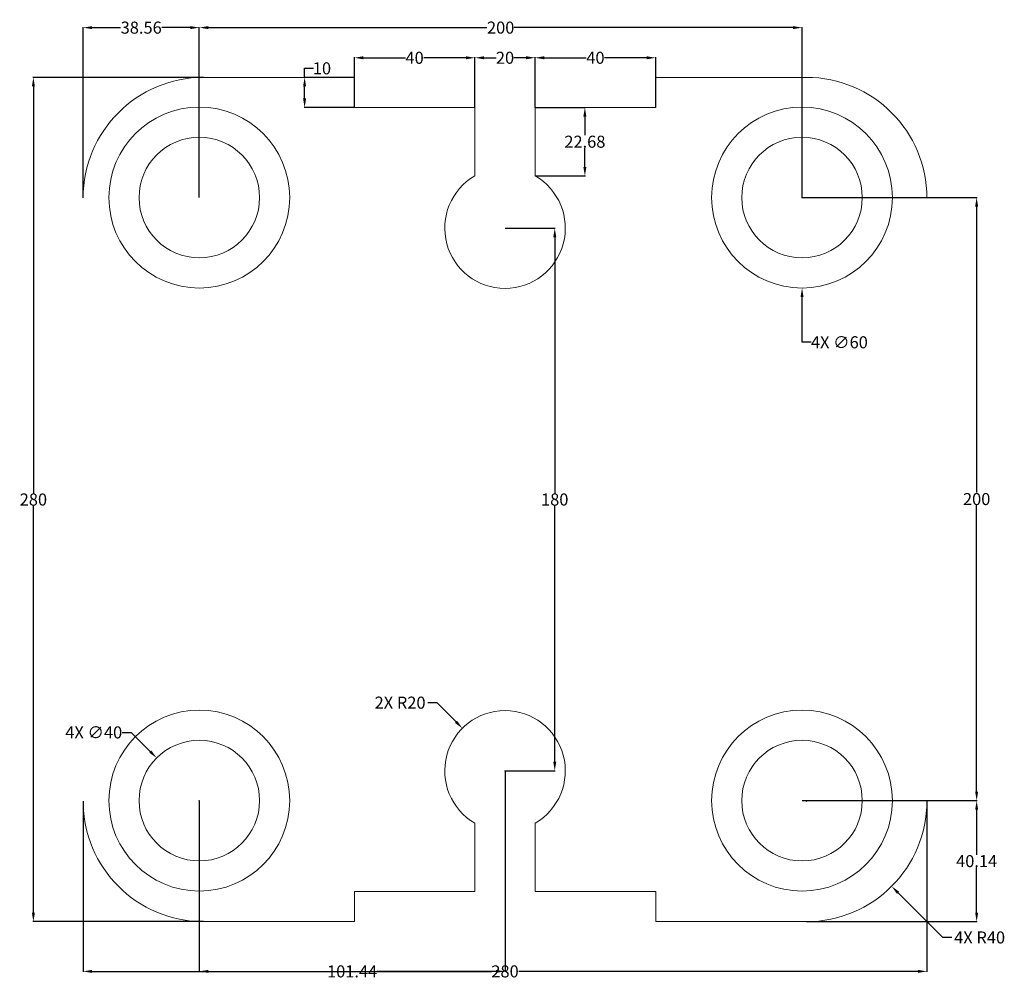
# Model space of a CAD drawing. Units: millimetres. Extents: x 803 to 1130, y 643 to 961.
import ezdxf

# ---------------------------------------------------------------- set-up
doc = ezdxf.new("R2010")
doc.units = ezdxf.units.MM
doc.header["$MEASUREMENT"] = 0
doc.layers.add('M-CONS', color=8, linetype='Continuous', lineweight=18)
doc.layers.add('M-DIMS', color=2, linetype='Continuous', lineweight=18)
doc.styles.get("Standard").update_dxf_attribs({"font": 'arial.ttf'})
doc.dimstyles.get("Standard").update_dxf_attribs({"dimtxt": 4, "dimasz": 3, "dimexe": 0.18, "dimexo": 0.0625, "dimgap": 0.09, "dimtad": 0, "dimtih": 1, "dimtoh": 1, "dimdec": 1, "dimzin": 0, "dimdsep": 46, "dimtxsty": 'Standard', "dimcen": 0.09, "dimadec": 0, "dimazin": 0, "dimtfac": 1, "dimtdec": 1, "dimtofl": 0, "dimtmove": 0, "dimatfit": 3, "dimfxl": 1, "dimtolj": 1, "dimtzin": 0, "dimarcsym": 0})

# ---------------------------------------------------------------- blocks, each defined once
blk = doc.blocks.new('MOUNT-BOSS-OD60-BORE40')
for radius in [30, 20]:
    blk.add_circle((0, 0, 20), radius)
blk = doc.blocks.new('*D2')
at = {"layer": 'Defpoints', "color": 0, "transparency": 16777216}
for p in [(823.97, 702.2), (1103.97, 702.2), (1103.97, 645.7)]:
    blk.add_point(p, dxfattribs=at)
at = {"layer": 'M-DIMS', "color": 0, "lineweight": -2, "transparency": 16777216}
for p, q in [((823.97, 702.14), (823.97, 645.52)), ((1103.97, 702.14), (1103.97, 645.52)), ((826.97, 645.7), (959.43, 645.7)), ((1100.97, 645.7), (968.51, 645.7))]:
    blk.add_line(p, q, dxfattribs=at)
at = {"layer": 'M-DIMS', "color": 0, "transparency": 16777216}
for points in [[(826.97, 646.2), (826.97, 645.2), (823.97, 645.7)], [(1100.97, 646.2), (1100.97, 645.2), (1103.97, 645.7)]]:
    blk.add_solid(points, dxfattribs=at)
at = {"layer": 'M-DIMS', "color": 0, "transparency": 16777216, "insert": (963.97, 645.7), "char_height": 4, "attachment_point": 5}
blk.add_mtext('\\A1;280', dxfattribs=at)
blk = doc.blocks.new('*D3')
at = {"layer": 'Defpoints', "color": 0, "transparency": 16777216}
for p in [(807.47, 942.2), (863.97, 942.2), (863.97, 662.2)]:
    blk.add_point(p, dxfattribs=at)
at = {"layer": 'M-DIMS', "color": 0, "lineweight": -2, "transparency": 16777216}
for p, q in [((863.91, 942.2), (807.29, 942.2)), ((807.47, 939.2), (807.47, 804.33)), ((807.47, 665.2), (807.47, 800.07)), ((863.91, 662.2), (807.29, 662.2))]:
    blk.add_line(p, q, dxfattribs=at)
at = {"layer": 'M-DIMS', "color": 0, "transparency": 16777216}
for points in [[(806.97, 939.2), (807.97, 939.2), (807.47, 942.2)], [(806.97, 665.2), (807.97, 665.2), (807.47, 662.2)]]:
    blk.add_solid(points, dxfattribs=at)
at = {"layer": 'M-DIMS', "color": 0, "transparency": 16777216, "insert": (807.47, 802.2), "char_height": 4, "attachment_point": 5}
blk.add_mtext('\\A1;280', dxfattribs=at)
blk = doc.blocks.new('*D4')
at = {"layer": 'Defpoints', "color": 0, "transparency": 16777216}
for p in [(1062.53, 958.7), (862.53, 902.34), (1062.53, 902.34)]:
    blk.add_point(p, dxfattribs=at)
at = {"layer": 'M-DIMS', "color": 0, "lineweight": -2, "transparency": 16777216}
for p, q in [((862.53, 902.4), (862.53, 958.88)), ((865.53, 958.7), (957.99, 958.7)), ((1059.53, 958.7), (967.06, 958.7)), ((1062.53, 902.4), (1062.53, 958.88))]:
    blk.add_line(p, q, dxfattribs=at)
at = {"layer": 'M-DIMS', "color": 0, "transparency": 16777216}
for points in [[(865.53, 959.2), (865.53, 958.2), (862.53, 958.7)], [(1059.53, 959.2), (1059.53, 958.2), (1062.53, 958.7)]]:
    blk.add_solid(points, dxfattribs=at)
at = {"layer": 'M-DIMS', "color": 0, "transparency": 16777216, "insert": (962.53, 958.7), "char_height": 4, "attachment_point": 5}
blk.add_mtext('\\A1;200', dxfattribs=at)
blk = doc.blocks.new('*D5')
at = {"layer": 'Defpoints', "color": 0, "transparency": 16777216}
for p in [(1062.53, 902.34), (1120.47, 902.34), (1062.53, 702.34)]:
    blk.add_point(p, dxfattribs=at)
at = {"layer": 'M-DIMS', "color": 0, "lineweight": -2, "transparency": 16777216}
for p, q in [((1062.59, 902.34), (1120.65, 902.34)), ((1120.47, 899.34), (1120.47, 804.47)), ((1120.47, 705.34), (1120.47, 800.21)), ((1062.59, 702.34), (1120.65, 702.34))]:
    blk.add_line(p, q, dxfattribs=at)
at = {"layer": 'M-DIMS', "color": 0, "transparency": 16777216}
for points in [[(1119.97, 899.34), (1120.97, 899.34), (1120.47, 902.34)], [(1119.97, 705.34), (1120.97, 705.34), (1120.47, 702.34)]]:
    blk.add_solid(points, dxfattribs=at)
at = {"layer": 'M-DIMS', "color": 0, "transparency": 16777216, "insert": (1120.47, 802.34), "char_height": 4, "attachment_point": 5}
blk.add_mtext('\\A1;200', dxfattribs=at)
blk = doc.blocks.new('*D6')
at = {"layer": 'Defpoints', "color": 0, "transparency": 16777216}
for p in [(862.53, 958.7), (823.97, 902.2), (862.53, 902.34)]:
    blk.add_point(p, dxfattribs=at)
at = {"layer": 'M-DIMS', "color": 0, "lineweight": -2, "transparency": 16777216}
for p, q in [((823.97, 902.26), (823.97, 958.88)), ((826.97, 958.7), (836.41, 958.7)), ((859.53, 958.7), (850.08, 958.7)), ((862.53, 902.4), (862.53, 958.88))]:
    blk.add_line(p, q, dxfattribs=at)
at = {"layer": 'M-DIMS', "color": 0, "transparency": 16777216}
for points in [[(826.97, 959.2), (826.97, 958.2), (823.97, 958.7)], [(859.53, 959.2), (859.53, 958.2), (862.53, 958.7)]]:
    blk.add_solid(points, dxfattribs=at)
at = {"layer": 'M-DIMS', "color": 0, "transparency": 16777216, "insert": (843.25, 958.7), "char_height": 4, "attachment_point": 5}
blk.add_mtext('\\A1;38.56', dxfattribs=at)
blk = doc.blocks.new('*D7')
at = {"layer": 'Defpoints', "color": 0, "transparency": 16777216}
for p in [(1062.53, 702.34), (1120.47, 702.34), (1063.97, 662.2)]:
    blk.add_point(p, dxfattribs=at)
at = {"layer": 'M-DIMS', "color": 0, "lineweight": -2, "transparency": 16777216}
for p, q in [((1062.59, 702.34), (1120.65, 702.34)), ((1120.47, 699.34), (1120.47, 684.4)), ((1120.47, 665.2), (1120.47, 680.14)), ((1064.03, 662.2), (1120.65, 662.2))]:
    blk.add_line(p, q, dxfattribs=at)
at = {"layer": 'M-DIMS', "color": 0, "transparency": 16777216}
for points in [[(1119.97, 699.34), (1120.97, 699.34), (1120.47, 702.34)], [(1119.97, 665.2), (1120.97, 665.2), (1120.47, 662.2)]]:
    blk.add_solid(points, dxfattribs=at)
at = {"layer": 'M-DIMS', "color": 0, "transparency": 16777216, "insert": (1120.47, 682.27), "char_height": 4, "attachment_point": 5}
blk.add_mtext('\\A1;40.14', dxfattribs=at)
blk = doc.blocks.new('*D8')
at = {"layer": 'Defpoints', "color": 0, "transparency": 16777216}
for p in [(963.97, 712.2), (862.53, 702.34), (963.97, 645.7)]:
    blk.add_point(p, dxfattribs=at)
at = {"layer": 'M-DIMS', "color": 0, "lineweight": -2, "transparency": 16777216}
for p, q in [((963.97, 712.14), (963.97, 645.52)), ((862.53, 702.28), (862.53, 645.52)), ((865.53, 645.7), (905.05, 645.7)), ((960.97, 645.7), (921.44, 645.7))]:
    blk.add_line(p, q, dxfattribs=at)
at = {"layer": 'M-DIMS', "color": 0, "transparency": 16777216}
for points in [[(865.53, 646.2), (865.53, 645.2), (862.53, 645.7)], [(960.97, 646.2), (960.97, 645.2), (963.97, 645.7)]]:
    blk.add_solid(points, dxfattribs=at)
at = {"layer": 'M-DIMS', "color": 0, "transparency": 16777216, "insert": (913.25, 645.7), "char_height": 4, "attachment_point": 5}
blk.add_mtext('\\A1;101.44', dxfattribs=at)
blk = doc.blocks.new('*D9')
at = {"layer": 'Defpoints', "color": 0, "transparency": 16777216}
for p in [(953.97, 948.7), (913.97, 932.2), (953.97, 932.2)]:
    blk.add_point(p, dxfattribs=at)
at = {"layer": 'M-DIMS', "color": 0, "lineweight": -2, "transparency": 16777216}
for p, q in [((913.97, 932.26), (913.97, 948.88)), ((916.97, 948.7), (930.94, 948.7)), ((950.97, 948.7), (937, 948.7)), ((953.97, 932.26), (953.97, 948.88))]:
    blk.add_line(p, q, dxfattribs=at)
at = {"layer": 'M-DIMS', "color": 0, "transparency": 16777216}
for points in [[(916.97, 949.2), (916.97, 948.2), (913.97, 948.7)], [(950.97, 949.2), (950.97, 948.2), (953.97, 948.7)]]:
    blk.add_solid(points, dxfattribs=at)
at = {"layer": 'M-DIMS', "color": 0, "transparency": 16777216, "insert": (933.97, 948.7), "char_height": 4, "attachment_point": 5}
blk.add_mtext('\\A1;40', dxfattribs=at)
blk = doc.blocks.new('*D10')
at = {"layer": 'Defpoints', "color": 0, "transparency": 16777216}
for p in [(973.97, 948.7), (953.97, 932.2), (973.97, 932.2)]:
    blk.add_point(p, dxfattribs=at)
at = {"layer": 'M-DIMS', "color": 0, "lineweight": -2, "transparency": 16777216}
for p, q in [((953.97, 932.26), (953.97, 948.88)), ((956.97, 948.7), (960.99, 948.7)), ((970.97, 948.7), (966.95, 948.7)), ((973.97, 932.26), (973.97, 948.88))]:
    blk.add_line(p, q, dxfattribs=at)
at = {"layer": 'M-DIMS', "color": 0, "transparency": 16777216}
for points in [[(956.97, 949.2), (956.97, 948.2), (953.97, 948.7)], [(970.97, 949.2), (970.97, 948.2), (973.97, 948.7)]]:
    blk.add_solid(points, dxfattribs=at)
at = {"layer": 'M-DIMS', "color": 0, "transparency": 16777216, "insert": (963.97, 948.7), "char_height": 4, "attachment_point": 5}
blk.add_mtext('\\A1;20', dxfattribs=at)
blk = doc.blocks.new('*D11')
at = {"layer": 'Defpoints', "color": 0, "transparency": 16777216}
for p in [(1013.97, 948.7), (973.97, 932.2), (1013.97, 932.2)]:
    blk.add_point(p, dxfattribs=at)
at = {"layer": 'M-DIMS', "color": 0, "lineweight": -2, "transparency": 16777216}
for p, q in [((973.97, 932.26), (973.97, 948.88)), ((976.97, 948.7), (990.94, 948.7)), ((1010.97, 948.7), (997, 948.7)), ((1013.97, 932.26), (1013.97, 948.88))]:
    blk.add_line(p, q, dxfattribs=at)
at = {"layer": 'M-DIMS', "color": 0, "transparency": 16777216}
for points in [[(976.97, 949.2), (976.97, 948.2), (973.97, 948.7)], [(1010.97, 949.2), (1010.97, 948.2), (1013.97, 948.7)]]:
    blk.add_solid(points, dxfattribs=at)
at = {"layer": 'M-DIMS', "color": 0, "transparency": 16777216, "insert": (993.97, 948.7), "char_height": 4, "attachment_point": 5}
blk.add_mtext('\\A1;40', dxfattribs=at)
blk = doc.blocks.new('*D12')
at = {"layer": 'Defpoints', "color": 0, "transparency": 16777216}
for p in [(897.47, 942.2), (913.97, 942.2), (913.97, 932.2)]:
    blk.add_point(p, dxfattribs=at)
at = {"layer": 'M-DIMS', "color": 0, "lineweight": -2, "transparency": 16777216}
for p, q in [((897.47, 942.2), (897.47, 945.2)), ((897.47, 945.2), (900.47, 945.2)), ((913.91, 942.2), (897.29, 942.2)), ((897.47, 935.2), (897.47, 939.2)), ((913.91, 932.2), (897.29, 932.2))]:
    blk.add_line(p, q, dxfattribs=at)
at = {"layer": 'M-DIMS', "color": 0, "transparency": 16777216}
for points in [[(896.97, 939.2), (897.97, 939.2), (897.47, 942.2)], [(896.97, 935.2), (897.97, 935.2), (897.47, 932.2)]]:
    blk.add_solid(points, dxfattribs=at)
at = {"layer": 'M-DIMS', "color": 0, "transparency": 16777216, "insert": (903.23, 945.2), "char_height": 4, "attachment_point": 5}
blk.add_mtext('\\A1;10', dxfattribs=at)
blk = doc.blocks.new('*D13')
at = {"layer": 'Defpoints', "color": 0, "transparency": 16777216}
for p in [(973.97, 932.2), (973.97, 909.52), (990.47, 909.52)]:
    blk.add_point(p, dxfattribs=at)
at = {"layer": 'M-DIMS', "color": 0, "lineweight": -2, "transparency": 16777216}
for p, q in [((974.03, 932.2), (990.65, 932.2)), ((990.47, 929.2), (990.47, 922.99)), ((990.47, 912.52), (990.47, 918.73)), ((974.03, 909.52), (990.65, 909.52))]:
    blk.add_line(p, q, dxfattribs=at)
at = {"layer": 'M-DIMS', "color": 0, "transparency": 16777216}
for points in [[(989.97, 929.2), (990.97, 929.2), (990.47, 932.2)], [(989.97, 912.52), (990.97, 912.52), (990.47, 909.52)]]:
    blk.add_solid(points, dxfattribs=at)
at = {"layer": 'M-DIMS', "color": 0, "transparency": 16777216, "insert": (990.47, 920.86), "char_height": 4, "attachment_point": 5}
blk.add_mtext('\\A1;22.68', dxfattribs=at)
blk = doc.blocks.new('*D14')
at = {"layer": 'Defpoints', "color": 0, "transparency": 16777216}
for p in [(963.97, 892.2), (963.97, 712.2), (980.47, 712.2)]:
    blk.add_point(p, dxfattribs=at)
at = {"layer": 'M-DIMS', "color": 0, "lineweight": -2, "transparency": 16777216}
for p, q in [((964.03, 892.2), (980.65, 892.2)), ((980.47, 889.2), (980.47, 804.33)), ((980.47, 715.2), (980.47, 800.07)), ((964.03, 712.2), (980.65, 712.2))]:
    blk.add_line(p, q, dxfattribs=at)
at = {"layer": 'M-DIMS', "color": 0, "transparency": 16777216}
for points in [[(979.97, 889.2), (980.97, 889.2), (980.47, 892.2)], [(979.97, 715.2), (980.97, 715.2), (980.47, 712.2)]]:
    blk.add_solid(points, dxfattribs=at)
at = {"layer": 'M-DIMS', "color": 0, "transparency": 16777216, "insert": (980.47, 802.2), "char_height": 4, "attachment_point": 5}
blk.add_mtext('\\A1;180', dxfattribs=at)
blk = doc.blocks.new('*D15')
at = {"layer": 'Defpoints', "color": 0, "transparency": 16777216}
for p in [(1063.97, 702.2), (1092.25, 673.92)]:
    blk.add_point(p, dxfattribs=at)
at = {"layer": 'M-DIMS', "color": 0, "lineweight": -2, "transparency": 16777216}
for p, q in [((1063.88, 702.2), (1064.06, 702.2)), ((1063.97, 702.11), (1063.97, 702.29)), ((1109.22, 656.95), (1094.38, 671.8)), ((1112.22, 656.95), (1109.22, 656.95))]:
    blk.add_line(p, q, dxfattribs=at)
at = {"layer": 'M-DIMS', "color": 0, "transparency": 16777216}
blk.add_solid([(1094.73, 672.15), (1094.02, 671.44), (1092.25, 673.92)], dxfattribs=at)
at = {"layer": 'M-DIMS', "color": 0, "transparency": 16777216, "insert": (1121.46, 656.95), "char_height": 4, "attachment_point": 5}
blk.add_mtext('\\A1;4X R40', dxfattribs=at)
blk = doc.blocks.new('*D16')
at = {"layer": 'Defpoints', "color": 0, "transparency": 16777216}
for p in [(1062.53, 932.34), (1062.53, 872.34)]:
    blk.add_point(p, dxfattribs=at)
at = {"layer": 'M-DIMS', "color": 0, "lineweight": -2, "transparency": 16777216}
for p, q in [((1062.44, 902.34), (1062.62, 902.34)), ((1062.53, 902.25), (1062.53, 902.43)), ((1062.53, 854.34), (1062.53, 869.34)), ((1065.53, 854.34), (1062.53, 854.34))]:
    blk.add_line(p, q, dxfattribs=at)
at = {"layer": 'M-DIMS', "color": 0, "transparency": 16777216}
blk.add_solid([(1063.03, 869.34), (1062.03, 869.34), (1062.53, 872.34)], dxfattribs=at)
at = {"layer": 'M-DIMS', "color": 0, "transparency": 16777216, "insert": (1074.92, 854.34), "char_height": 4, "attachment_point": 5}
blk.add_mtext('\\A1;4X ∅60', dxfattribs=at)
blk = doc.blocks.new('*D17')
at = {"layer": 'Defpoints', "color": 0, "transparency": 16777216}
for p in [(848.38, 716.48), (876.67, 688.2)]:
    blk.add_point(p, dxfattribs=at)
at = {"layer": 'M-DIMS', "color": 0, "lineweight": -2, "transparency": 16777216}
for p, q in [((836.9, 724.96), (839.9, 724.96)), ((839.9, 724.96), (846.26, 718.6)), ((862.44, 702.34), (862.62, 702.34)), ((862.53, 702.25), (862.53, 702.43))]:
    blk.add_line(p, q, dxfattribs=at)
at = {"layer": 'M-DIMS', "color": 0, "transparency": 16777216}
blk.add_solid([(846.61, 718.95), (845.91, 718.25), (848.38, 716.48)], dxfattribs=at)
at = {"layer": 'M-DIMS', "color": 0, "transparency": 16777216, "insert": (827.5, 724.96), "char_height": 4, "attachment_point": 5}
blk.add_mtext('\\A1;4X ∅40', dxfattribs=at)
blk = doc.blocks.new('*D18')
at = {"layer": 'Defpoints', "color": 0, "transparency": 16777216}
for p in [(949.83, 726.34), (963.97, 712.2)]:
    blk.add_point(p, dxfattribs=at)
at = {"layer": 'M-DIMS', "color": 0, "lineweight": -2, "transparency": 16777216}
for p, q in [((938.34, 734.83), (941.34, 734.83)), ((941.34, 734.83), (947.71, 728.47)), ((963.97, 712.11), (963.97, 712.29)), ((963.88, 712.2), (964.06, 712.2))]:
    blk.add_line(p, q, dxfattribs=at)
at = {"layer": 'M-DIMS', "color": 0, "transparency": 16777216}
blk.add_solid([(948.06, 728.82), (947.35, 728.11), (949.83, 726.34)], dxfattribs=at)
at = {"layer": 'M-DIMS', "color": 0, "transparency": 16777216, "insert": (929.15, 734.83), "char_height": 4, "attachment_point": 5}
blk.add_mtext('\\A1;2X R20', dxfattribs=at)

msp = doc.modelspace()

# ---------------------------------------------------------------- linework, layer by layer
at = {"layer": 'M-CONS'}
for p, q in [((863.97, 942.202), (913.97, 942.202)), ((913.97, 932.202), (913.97, 942.202)), ((1013.97, 932.202), (1013.97, 942.202)), ((1013.97, 942.202), (1063.97, 942.202)), ((953.97, 932.202), (913.97, 932.202)), ((953.97, 932.202), (953.97, 909.522)), ((973.97, 932.202), (973.97, 909.522)), ((1013.97, 932.202), (973.97, 932.202)), ((953.97, 672.202), (953.97, 694.881)), ((973.97, 672.202), (973.97, 694.881)), ((913.97, 672.202), (913.97, 662.202)), ((953.97, 672.202), (913.97, 672.202)), ((1013.97, 672.202), (973.97, 672.202)), ((1013.97, 672.202), (1013.97, 662.202)), ((913.97, 662.202), (863.97, 662.202)), ((1063.97, 662.202), (1013.97, 662.202))]:
    msp.add_line(p, q, dxfattribs=at)
for centre, radius, start, end in [((863.97, 902.202), 40, 90, 180), ((1063.97, 902.202), 40, 0, 90), ((963.97, 892.202), 20, 120, 60), ((963.97, 712.202), 20, 300, 240), ((863.97, 702.202), 40, 180, 270), ((1063.97, 702.202), 40, 270, 0)]:
    msp.add_arc(centre, radius, start, end, dxfattribs=at)

# ---------------------------------------------------------------- block references
for p in [(862.526, 902.338), (1062.526, 902.338), (862.526, 702.338), (1062.526, 702.338)]:
    msp.add_blockref('MOUNT-BOSS-OD60-BORE40', p, dxfattribs=at)

# ---------------------------------------------------------------- dimensions: what is measured, and where the dimension line sits
at = {"layer": 'M-DIMS'}
for base, p1, p2, override, picture, middle in [((862.526, 958.702), (823.97, 902.202), (862.526, 902.338), {"dimdec": 2, "dimlfac": 1, "dimrnd": 0, "dimzin": 0, "dimdsep": 46, "dimlunit": 2}, '*D6', (843.248, 958.702)), ((1062.526, 958.702), (862.526, 902.338), (1062.526, 902.338), {"dimdec": 0, "dimlfac": 1, "dimrnd": 0, "dimzin": 0, "dimdsep": 46, "dimlunit": 2}, '*D4', (962.526, 958.702)), ((953.97, 948.702), (913.97, 932.202), (953.97, 932.202), {"dimdec": 0, "dimlfac": 1, "dimrnd": 0, "dimzin": 0, "dimdsep": 46, "dimlunit": 2}, '*D9', (933.97, 948.702)), ((973.97, 948.702), (953.97, 932.202), (973.97, 932.202), {"dimdec": 0, "dimlfac": 1, "dimrnd": 0, "dimzin": 0, "dimdsep": 46, "dimlunit": 2}, '*D10', (963.97, 948.702)), ((1013.97, 948.702), (973.97, 932.202), (1013.97, 932.202), {"dimdec": 0, "dimlfac": 1, "dimrnd": 0, "dimzin": 0, "dimdsep": 46, "dimlunit": 2}, '*D11', (993.97, 948.702)), ((963.97, 645.702), (862.526, 702.338), (963.97, 712.202), {"dimdec": 2, "dimlfac": 1, "dimrnd": 0, "dimzin": 0, "dimdsep": 46, "dimlunit": 2}, '*D8', (913.248, 645.702)), ((1103.97, 645.702), (823.97, 702.202), (1103.97, 702.202), {"dimdec": 0, "dimlfac": 1, "dimrnd": 0, "dimzin": 0, "dimdsep": 46, "dimlunit": 2}, '*D2', (963.97, 645.702))]:
    dim = msp.add_linear_dim(base=base, p1=p1, p2=p2, dimstyle='Standard', override=override, dxfattribs=at)
    dim.commit()
    dim.dimension.update_dxf_attribs({"geometry": picture, "text_midpoint": middle})
for base, p1, p2, angle, override, picture, middle in [((897.47, 942.202), (913.97, 932.202), (913.97, 942.202), 90, {"dimdec": 0, "dimlfac": 1, "dimrnd": 0, "dimzin": 0, "dimdsep": 46, "dimlunit": 2}, '*D12', (903.23, 945.202)), ((807.47, 942.202), (863.97, 662.202), (863.97, 942.202), 90, {"dimdec": 0, "dimlfac": 1, "dimrnd": 0, "dimzin": 0, "dimdsep": 46, "dimlunit": 2}, '*D3', (807.47, 802.202)), ((990.47, 909.522), (973.97, 932.202), (973.97, 909.522), 270, {"dimdec": 2, "dimlfac": 1, "dimrnd": 0, "dimzin": 0, "dimdsep": 46, "dimlunit": 2}, '*D13', (990.47, 920.862)), ((1120.47, 902.338), (1062.526, 702.338), (1062.526, 902.338), 90, {"dimdec": 0, "dimlfac": 1, "dimrnd": 0, "dimzin": 0, "dimdsep": 46, "dimlunit": 2}, '*D5', (1120.47, 802.338)), ((980.47, 712.202), (963.97, 892.202), (963.97, 712.202), 270, {"dimdec": 0, "dimlfac": 1, "dimrnd": 0, "dimzin": 0, "dimdsep": 46, "dimlunit": 2}, '*D14', (980.47, 802.202)), ((1120.47, 702.338), (1063.97, 662.202), (1062.526, 702.338), 90, {"dimdec": 2, "dimlfac": 1, "dimrnd": 0, "dimzin": 0, "dimdsep": 46, "dimlunit": 2}, '*D7', (1120.47, 682.27))]:
    dim = msp.add_linear_dim(base=base, p1=p1, p2=p2, angle=angle, dimstyle='Standard', override=override, dxfattribs=at)
    dim.commit()
    dim.dimension.update_dxf_attribs({"geometry": picture, "text_midpoint": middle})
for p1, p2, picture, middle in [((1062.526, 932.338), (1062.526, 872.338), '*D16', (1074.922, 854.338)), ((876.67, 688.198), (848.382, 716.478), '*D17', (827.5, 724.962))]:
    dim = msp.add_diameter_dim_2p(p1=p1, p2=p2, text='4X <>', dimstyle='Standard', override={"dimdec": 0, "dimlfac": 1, "dimrnd": 0, "dimzin": 0, "dimdsep": 46, "dimlunit": 2}, dxfattribs=at)
    dim.commit()
    dim.dimension.update_dxf_attribs({"geometry": picture, "text_midpoint": middle, "dimtype": 163})
for center, mpoint, text, picture, middle in [((963.97, 712.202), (949.828, 726.344), '2X <>', '*D18', (929.149, 734.83)), ((1063.97, 702.202), (1092.254, 673.918), '4X <>', '*D15', (1121.465, 656.947))]:
    dim = msp.add_radius_dim(center=center, mpoint=mpoint, text=text, dimstyle='Standard', override={"dimdec": 0, "dimlfac": 1, "dimrnd": 0, "dimzin": 0, "dimdsep": 46, "dimlunit": 2}, dxfattribs=at)
    dim.commit()
    dim.dimension.update_dxf_attribs({"geometry": picture, "text_midpoint": middle, "dimtype": 164})

doc.saveas('drawing.dxf')
